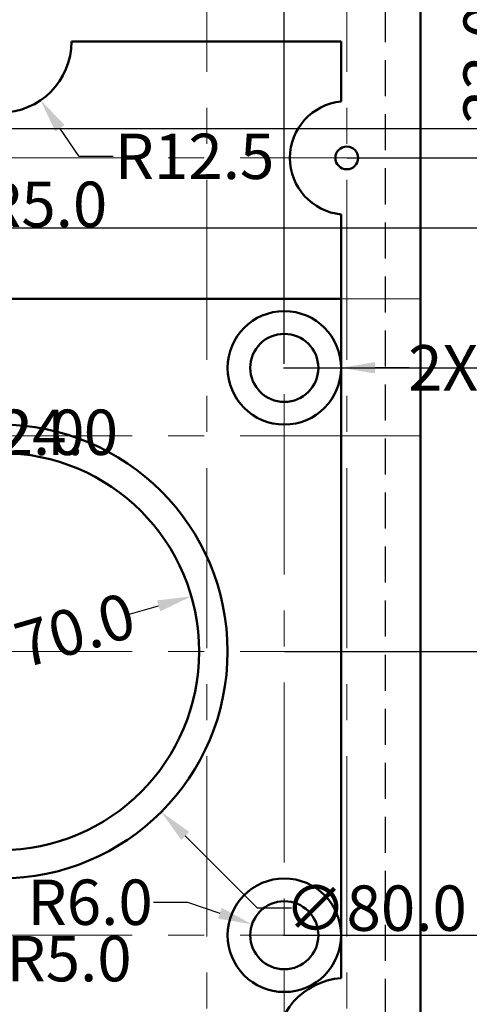
# Model space of a CAD drawing. Units: inches. Extents: x 11765 to 12471, y 10149 to 10793.
# Tile 5 of 8: x 11996 to 12076, y 10530 to 10704. Entities that reach past the tile are written whole.
import ezdxf

# ---------------------------------------------------------------- set-up
doc = ezdxf.new("R2010")
doc.units = ezdxf.units.IN
doc.header["$MEASUREMENT"] = 0
doc.linetypes.add('CENTER', pattern=[50.8, 31.75, -6.35, 6.35, -6.35])
doc.linetypes.add('HIDDEN', pattern=[9.525, 6.35, -3.175])
for name, color, linetype, lineweight in [('M-CNTR', 30, 'CENTER', 18), ('M-DIMS', 2, 'Continuous', 25), ('M-HIDN', 41, 'HIDDEN', 25), ('M-OUTL', 7, 'Continuous', 50)]:
    doc.layers.add(name, color=color, linetype=linetype, lineweight=lineweight)
doc.styles.get("Standard").update_dxf_attribs({"font": 'arial.ttf'})
doc.dimstyles.get("Standard").update_dxf_attribs({"dimtxt": 8, "dimasz": 6, "dimexe": 0.18, "dimexo": 0.0625, "dimgap": 0.09, "dimtad": 0, "dimtoh": 1, "dimdec": 1, "dimzin": 0, "dimdsep": 46, "dimtxsty": 'Standard', "dimcen": 0.09, "dimadec": 0, "dimazin": 0, "dimtfac": 1, "dimtdec": 1, "dimtofl": 0, "dimtmove": 0, "dimatfit": 3, "dimfxl": 1, "dimtolj": 1, "dimtzin": 0, "dimarcsym": 0})

# ---------------------------------------------------------------- blocks, each defined once
blk = doc.blocks.new('*D5')
at = {"layer": 'Defpoints', "color": 0, "transparency": 16777216}
for p in [(11992.91, 10750.5), (11992.91, 10699.65), (12042.91, 10642.79)]:
    blk.add_point(p, dxfattribs=at)
at = {"layer": 'M-DIMS', "color": 0, "lineweight": -2, "transparency": 16777216}
for p, q in [((11992.91, 10699.71), (11992.91, 10750.68)), ((11998.91, 10750.5), (12007.45, 10750.5)), ((12036.91, 10750.5), (12028.38, 10750.5)), ((12042.91, 10642.86), (12042.91, 10750.68))]:
    blk.add_line(p, q, dxfattribs=at)
at = {"layer": 'M-DIMS', "color": 0, "transparency": 16777216}
for points in [[(11998.91, 10751.5), (11998.91, 10749.5), (11992.91, 10750.5)], [(12036.91, 10751.5), (12036.91, 10749.5), (12042.91, 10750.5)]]:
    blk.add_solid(points, dxfattribs=at)
at = {"layer": 'M-DIMS', "color": 0, "transparency": 16777216, "insert": (12017.91, 10750.5), "char_height": 8, "attachment_point": 5}
blk.add_mtext('\\A1;50.0', dxfattribs=at)
blk = doc.blocks.new('*D7')
at = {"layer": 'Defpoints', "color": 0, "transparency": 16777216}
for p in [(12066.91, 10679.15), (12145.22, 10679.15), (12066.91, 10592.15)]:
    blk.add_point(p, dxfattribs=at)
at = {"layer": 'M-DIMS', "color": 0, "lineweight": -2, "transparency": 16777216}
for p, q in [((12066.97, 10679.15), (12145.4, 10679.15)), ((12145.22, 10673.15), (12145.22, 10646.12)), ((12145.22, 10598.15), (12145.22, 10625.17)), ((12066.97, 10592.15), (12145.4, 10592.15))]:
    blk.add_line(p, q, dxfattribs=at)
at = {"layer": 'M-DIMS', "color": 0, "transparency": 16777216}
for points in [[(12144.22, 10673.15), (12146.22, 10673.15), (12145.22, 10679.15)], [(12144.22, 10598.15), (12146.22, 10598.15), (12145.22, 10592.15)]]:
    blk.add_solid(points, dxfattribs=at)
at = {"layer": 'M-DIMS', "color": 0, "transparency": 16777216, "insert": (12145.22, 10635.65), "char_height": 8, "attachment_point": 5, "rotation": 90}
blk.add_mtext('\\A1;87.0', dxfattribs=at)
blk = doc.blocks.new('*D8')
at = {"layer": 'Defpoints', "color": 0, "transparency": 16777216}
for p in [(12042.91, 10642.15), (12042.91, 10592.15), (12085.66, 10592.15)]:
    blk.add_point(p, dxfattribs=at)
at = {"layer": 'M-DIMS', "color": 0, "lineweight": -2, "transparency": 16777216}
for p, q in [((12042.97, 10642.15), (12085.84, 10642.15)), ((12085.66, 10636.15), (12085.66, 10627.61)), ((12085.66, 10598.15), (12085.66, 10606.68)), ((12042.97, 10592.15), (12085.84, 10592.15))]:
    blk.add_line(p, q, dxfattribs=at)
at = {"layer": 'M-DIMS', "color": 0, "transparency": 16777216}
for points in [[(12084.66, 10636.15), (12086.66, 10636.15), (12085.66, 10642.15)], [(12084.66, 10598.15), (12086.66, 10598.15), (12085.66, 10592.15)]]:
    blk.add_solid(points, dxfattribs=at)
at = {"layer": 'M-DIMS', "color": 0, "transparency": 16777216, "insert": (12085.66, 10617.15), "char_height": 8, "attachment_point": 5, "rotation": 90}
blk.add_mtext('\\A1;50.0', dxfattribs=at)
blk = doc.blocks.new('*D9')
at = {"layer": 'Defpoints', "color": 0, "transparency": 16777216}
for p in [(12042.91, 10592.15), (12085.66, 10592.15), (12042.91, 10542.15)]:
    blk.add_point(p, dxfattribs=at)
at = {"layer": 'M-DIMS', "color": 0, "lineweight": -2, "transparency": 16777216}
for p, q in [((12042.97, 10592.15), (12085.84, 10592.15)), ((12085.66, 10586.15), (12085.66, 10577.61)), ((12085.66, 10548.15), (12085.66, 10556.68)), ((12042.97, 10542.15), (12085.84, 10542.15))]:
    blk.add_line(p, q, dxfattribs=at)
at = {"layer": 'M-DIMS', "color": 0, "transparency": 16777216}
for points in [[(12084.66, 10586.15), (12086.66, 10586.15), (12085.66, 10592.15)], [(12084.66, 10548.15), (12086.66, 10548.15), (12085.66, 10542.15)]]:
    blk.add_solid(points, dxfattribs=at)
at = {"layer": 'M-DIMS', "color": 0, "transparency": 16777216, "insert": (12085.66, 10567.15), "char_height": 8, "attachment_point": 5, "rotation": 90}
blk.add_mtext('\\A1;50.0', dxfattribs=at)
blk = doc.blocks.new('*D12')
at = {"layer": 'Defpoints', "color": 0, "transparency": 16777216}
for p in [(12130.14, 10592.15), (12029.23, 10443.15), (12167.12, 10443.15)]:
    blk.add_point(p, dxfattribs=at)
at = {"layer": 'M-DIMS', "color": 0, "lineweight": -2, "transparency": 16777216}
for p, q in [((12130.2, 10592.15), (12167.3, 10592.15)), ((12167.12, 10586.15), (12167.12, 10530.84)), ((12167.12, 10449.15), (12167.12, 10504.45)), ((12029.29, 10443.15), (12167.3, 10443.15))]:
    blk.add_line(p, q, dxfattribs=at)
at = {"layer": 'M-DIMS', "color": 0, "transparency": 16777216}
for points in [[(12166.12, 10586.15), (12168.12, 10586.15), (12167.12, 10592.15)], [(12166.12, 10449.15), (12168.12, 10449.15), (12167.12, 10443.15)]]:
    blk.add_solid(points, dxfattribs=at)
at = {"layer": 'M-DIMS', "color": 0, "transparency": 16777216, "insert": (12167.12, 10517.65), "char_height": 8, "attachment_point": 5, "rotation": 90}
blk.add_mtext('\\A1;149.0', dxfattribs=at)
blk = doc.blocks.new('*D14')
at = {"layer": 'Defpoints', "color": 0, "transparency": 16777216}
for p in [(12156.23, 10592.15), (12216.5, 10592.15), (11992.91, 10372.15)]:
    blk.add_point(p, dxfattribs=at)
at = {"layer": 'M-DIMS', "color": 0, "lineweight": -2, "transparency": 16777216}
for p, q in [((12156.3, 10592.15), (12216.68, 10592.15)), ((12216.5, 10586.15), (12216.5, 10495.79)), ((12216.5, 10378.15), (12216.5, 10468.5)), ((11992.97, 10372.15), (12216.68, 10372.15))]:
    blk.add_line(p, q, dxfattribs=at)
at = {"layer": 'M-DIMS', "color": 0, "transparency": 16777216}
for points in [[(12215.5, 10586.15), (12217.5, 10586.15), (12216.5, 10592.15)], [(12215.5, 10378.15), (12217.5, 10378.15), (12216.5, 10372.15)]]:
    blk.add_solid(points, dxfattribs=at)
at = {"layer": 'M-DIMS', "color": 0, "transparency": 16777216, "insert": (12216.5, 10482.15), "char_height": 8, "attachment_point": 5, "rotation": 90}
blk.add_mtext('\\A1;220.0', dxfattribs=at)
blk = doc.blocks.new('*D28')
at = {"layer": 'Defpoints', "color": 0, "transparency": 16777216}
for p in [(12053.91, 10712.15), (12078.49, 10712.15), (12053.91, 10679.15)]:
    blk.add_point(p, dxfattribs=at)
at = {"layer": 'M-DIMS', "color": 0, "lineweight": -2, "transparency": 16777216}
for p, q in [((12078.49, 10718.15), (12078.49, 10724.15)), ((12053.97, 10712.15), (12078.67, 10712.15)), ((12053.97, 10679.15), (12078.67, 10679.15)), ((12078.49, 10673.15), (12078.49, 10667.15))]:
    blk.add_line(p, q, dxfattribs=at)
at = {"layer": 'M-DIMS', "color": 0, "transparency": 16777216}
for points in [[(12077.49, 10718.15), (12079.49, 10718.15), (12078.49, 10712.15)], [(12077.49, 10673.15), (12079.49, 10673.15), (12078.49, 10679.15)]]:
    blk.add_solid(points, dxfattribs=at)
at = {"layer": 'M-DIMS', "color": 0, "transparency": 16777216, "insert": (12078.49, 10695.65), "char_height": 8, "attachment_point": 5, "rotation": 90}
blk.add_mtext('\\A1;33.0', dxfattribs=at)
blk = doc.blocks.new('*D33')
at = {"layer": 'Defpoints', "color": 0, "transparency": 16777216}
for p in [(11992.91, 10699.65), (11999.97, 10689.33)]:
    blk.add_point(p, dxfattribs=at)
at = {"layer": 'M-DIMS', "color": 0, "lineweight": -2, "transparency": 16777216}
for p, q in [((11992.82, 10699.65), (11993, 10699.65)), ((11992.91, 10699.56), (11992.91, 10699.74)), ((12006.75, 10679.43), (12003.36, 10684.38)), ((12012.75, 10679.43), (12006.75, 10679.43))]:
    blk.add_line(p, q, dxfattribs=at)
at = {"layer": 'M-DIMS', "color": 0, "transparency": 16777216}
blk.add_solid([(12004.19, 10684.95), (12002.54, 10683.82), (11999.97, 10689.33)], dxfattribs=at)
at = {"layer": 'M-DIMS', "color": 0, "transparency": 16777216, "insert": (12027.09, 10679.43), "char_height": 8, "attachment_point": 5}
blk.add_mtext('\\A1;R12.5', dxfattribs=at)
blk = doc.blocks.new('*D34')
at = {"layer": 'Defpoints', "color": 0, "transparency": 16777216}
for p in [(11969.55, 10659.29), (11965.72, 10656.07)]:
    blk.add_point(p, dxfattribs=at)
at = {"layer": 'M-DIMS', "color": 0, "lineweight": -2, "transparency": 16777216}
for p, q in [((11983.49, 10670.97), (11970.32, 10659.93)), ((11989.49, 10670.97), (11983.49, 10670.97))]:
    blk.add_line(p, q, dxfattribs=at)
at = {"layer": 'M-DIMS', "color": 0, "transparency": 16777216}
blk.add_solid([(11969.68, 10660.69), (11970.96, 10659.16), (11965.72, 10656.07)], dxfattribs=at)
at = {"layer": 'M-DIMS', "color": 0, "transparency": 16777216, "insert": (12000.68, 10670.97), "char_height": 8, "attachment_point": 5}
blk.add_mtext('\\A1;R5.0', dxfattribs=at)
blk = doc.blocks.new('*D41')
at = {"layer": 'Defpoints', "color": 0, "transparency": 16777216}
for p in [(11987.78, 10526.02), (11987.78, 10521.02)]:
    blk.add_point(p, dxfattribs=at)
at = {"layer": 'M-DIMS', "color": 0, "lineweight": -2, "transparency": 16777216}
for p, q in [((11993.78, 10538.02), (11987.78, 10538.02)), ((11987.78, 10538.02), (11987.78, 10532.02)), ((11987.69, 10521.02), (11987.87, 10521.02)), ((11987.78, 10520.93), (11987.78, 10521.11))]:
    blk.add_line(p, q, dxfattribs=at)
at = {"layer": 'M-DIMS', "color": 0, "transparency": 16777216}
blk.add_solid([(11986.78, 10532.02), (11988.78, 10532.02), (11987.78, 10526.02)], dxfattribs=at)
at = {"layer": 'M-DIMS', "color": 0, "transparency": 16777216, "insert": (12004.97, 10538.02), "char_height": 8, "attachment_point": 5}
blk.add_mtext('\\A1;R5.0', dxfattribs=at)
blk = doc.blocks.new('*D42')
at = {"layer": 'Defpoints', "color": 0, "transparency": 16777216}
for p in [(12026.53, 10601.87), (11959.29, 10582.42)]:
    blk.add_point(p, dxfattribs=at)
at = {"layer": 'M-DIMS', "color": 0, "lineweight": -2, "transparency": 16777216}
blk.add_line((12015.01, 10598.54), (12020.77, 10600.2), dxfattribs=at)
at = {"layer": 'M-DIMS', "color": 0, "transparency": 16777216}
blk.add_solid([(12020.49, 10601.16), (12021.05, 10599.24), (12026.53, 10601.87)], dxfattribs=at)
at = {"layer": 'M-DIMS', "color": 0, "transparency": 16777216, "insert": (12000.77, 10594.42), "char_height": 8, "attachment_point": 5, "rotation": 16.1306}
blk.add_mtext('\\A1;∅70.0', dxfattribs=at)
blk = doc.blocks.new('*D43')
at = {"layer": 'Defpoints', "color": 0, "transparency": 16777216}
for p in [(11953.39, 10598.33), (12032.43, 10585.96)]:
    blk.add_point(p, dxfattribs=at)
at = {"layer": 'M-DIMS', "color": 0, "lineweight": -2, "transparency": 16777216}
for p, q in [((11927.12, 10602.44), (11947.47, 10599.26)), ((11992.82, 10592.15), (11993, 10592.15)), ((11992.91, 10592.06), (11992.91, 10592.24))]:
    blk.add_line(p, q, dxfattribs=at)
at = {"layer": 'M-DIMS', "color": 0, "transparency": 16777216}
blk.add_solid([(11947.62, 10600.25), (11947.31, 10598.27), (11953.39, 10598.33)], dxfattribs=at)
at = {"layer": 'M-DIMS', "color": 0, "transparency": 16777216, "insert": (11912.3, 10602.44), "char_height": 8, "attachment_point": 5}
blk.add_mtext('\\A1;∅80.0', dxfattribs=at)
blk = doc.blocks.new('*D49')
at = {"layer": 'Defpoints', "color": 0, "transparency": 16777216}
for p in [(12037.23, 10544.08), (12042.91, 10542.15)]:
    blk.add_point(p, dxfattribs=at)
at = {"layer": 'M-DIMS', "color": 0, "lineweight": -2, "transparency": 16777216}
for p, q in [((12019.88, 10547.96), (12025.88, 10547.96)), ((12025.88, 10547.96), (12031.55, 10546.02)), ((12042.82, 10542.15), (12043, 10542.15)), ((12042.91, 10542.06), (12042.91, 10542.24))]:
    blk.add_line(p, q, dxfattribs=at)
at = {"layer": 'M-DIMS', "color": 0, "transparency": 16777216}
blk.add_solid([(12031.88, 10546.97), (12031.23, 10545.07), (12037.23, 10544.08)], dxfattribs=at)
at = {"layer": 'M-DIMS', "color": 0, "transparency": 16777216, "insert": (12008.69, 10547.96), "char_height": 8, "attachment_point": 5}
blk.add_mtext('\\A1;R6.0', dxfattribs=at)
blk = doc.blocks.new('*D62')
at = {"layer": 'Defpoints', "color": 0, "transparency": 16777216}
for p in [(12379.9, 10706.15), (11848.16, 10684.29), (12385.4, 10684.29)]:
    blk.add_point(p, dxfattribs=at)
at = {"layer": 'M-DIMS', "color": 0, "lineweight": -2, "transparency": 16777216}
for p, q in [((12379.83, 10706.15), (11847.98, 10706.15)), ((11848.16, 10700.15), (11848.16, 10690.29)), ((12385.33, 10684.29), (11847.98, 10684.29)), ((11848.16, 10684.29), (11848.16, 10678.29)), ((11848.16, 10678.29), (11842.16, 10678.29))]:
    blk.add_line(p, q, dxfattribs=at)
at = {"layer": 'M-DIMS', "color": 0, "transparency": 16777216}
for points in [[(11847.16, 10700.15), (11849.16, 10700.15), (11848.16, 10706.15)], [(11847.16, 10690.29), (11849.16, 10690.29), (11848.16, 10684.29)]]:
    blk.add_solid(points, dxfattribs=at)
at = {"layer": 'M-DIMS', "color": 0, "transparency": 16777216, "insert": (11828.51, 10678.29), "char_height": 8, "attachment_point": 5}
blk.add_mtext('\\A1;21.86', dxfattribs=at)
blk = doc.blocks.new('*D63')
at = {"layer": 'Defpoints', "color": 0, "transparency": 16777216}
for p in [(12385.4, 10684.29), (11848.16, 10666.79), (12385.4, 10666.79)]:
    blk.add_point(p, dxfattribs=at)
at = {"layer": 'M-DIMS', "color": 0, "lineweight": -2, "transparency": 16777216}
for p, q in [((12385.33, 10684.29), (11847.98, 10684.29)), ((11848.16, 10678.29), (11848.16, 10672.79)), ((12385.33, 10666.79), (11847.98, 10666.79)), ((11848.16, 10666.79), (11848.16, 10660.79)), ((11848.16, 10660.79), (11842.16, 10660.79))]:
    blk.add_line(p, q, dxfattribs=at)
at = {"layer": 'M-DIMS', "color": 0, "transparency": 16777216}
for points in [[(11847.16, 10678.29), (11849.16, 10678.29), (11848.16, 10684.29)], [(11847.16, 10672.79), (11849.16, 10672.79), (11848.16, 10666.79)]]:
    blk.add_solid(points, dxfattribs=at)
at = {"layer": 'M-DIMS', "color": 0, "transparency": 16777216, "insert": (11832.03, 10660.79), "char_height": 8, "attachment_point": 5}
blk.add_mtext('\\A1;17.5', dxfattribs=at)
blk = doc.blocks.new('*D68')
at = {"layer": 'Defpoints', "color": 0, "transparency": 16777216}
for p in [(11964.61, 10620.41), (12021.22, 10563.88)]:
    blk.add_point(p, dxfattribs=at)
at = {"layer": 'M-DIMS', "color": 0, "lineweight": -2, "transparency": 16777216}
for p, q in [((11992.82, 10592.15), (11993, 10592.15)), ((11992.91, 10592.06), (11992.91, 10592.24)), ((12038.2, 10546.92), (12025.46, 10559.64)), ((12044.2, 10546.92), (12038.2, 10546.92))]:
    blk.add_line(p, q, dxfattribs=at)
at = {"layer": 'M-DIMS', "color": 0, "transparency": 16777216}
blk.add_solid([(12026.17, 10560.35), (12024.76, 10558.94), (12021.22, 10563.88)], dxfattribs=at)
at = {"layer": 'M-DIMS', "color": 0, "transparency": 16777216, "insert": (12059.02, 10546.92), "char_height": 8, "attachment_point": 5}
blk.add_mtext('\\A1;∅80.0', dxfattribs=at)
blk = doc.blocks.new('*D69')
at = {"layer": 'Defpoints', "color": 0, "transparency": 16777216}
for p in [(11968.18, 10616.92), (12017.64, 10567.38)]:
    blk.add_point(p, dxfattribs=at)
at = {"layer": 'M-DIMS', "color": 0, "lineweight": -2, "transparency": 16777216}
for p, q in [((11947.35, 10631.78), (11953.35, 10631.78)), ((11953.35, 10631.78), (11963.95, 10621.16)), ((11992.82, 10592.15), (11993, 10592.15)), ((11992.91, 10592.06), (11992.91, 10592.24))]:
    blk.add_line(p, q, dxfattribs=at)
at = {"layer": 'M-DIMS', "color": 0, "transparency": 16777216}
blk.add_solid([(11964.65, 10621.87), (11963.24, 10620.46), (11968.18, 10616.92)], dxfattribs=at)
at = {"layer": 'M-DIMS', "color": 0, "transparency": 16777216, "insert": (11932.53, 10631.78), "char_height": 8, "attachment_point": 5}
blk.add_mtext('\\A1;∅70.0', dxfattribs=at)
blk = doc.blocks.new('*D78')
at = {"layer": 'Defpoints', "color": 0, "transparency": 16777216}
for p in [(11930.91, 10630.79), (11954.91, 10630.79)]:
    blk.add_point(p, dxfattribs=at)
at = {"layer": 'M-DIMS', "color": 0, "lineweight": -2, "transparency": 16777216}
for p, q in [((11942.82, 10630.79), (11943, 10630.79)), ((11942.91, 10630.7), (11942.91, 10630.88)), ((11966.91, 10630.79), (11960.91, 10630.79))]:
    blk.add_line(p, q, dxfattribs=at)
at = {"layer": 'M-DIMS', "color": 0, "transparency": 16777216}
blk.add_solid([(11960.91, 10631.79), (11960.91, 10629.79), (11954.91, 10630.79)], dxfattribs=at)
at = {"layer": 'M-DIMS', "color": 0, "transparency": 16777216, "insert": (11990.18, 10630.79), "char_height": 8, "attachment_point": 5}
blk.add_mtext('\\A1;2X ∅24.0', dxfattribs=at)
blk = doc.blocks.new('*D80')
at = {"layer": 'Defpoints', "color": 0, "transparency": 16777216}
for p in [(12032.91, 10642.15), (12052.91, 10642.15)]:
    blk.add_point(p, dxfattribs=at)
at = {"layer": 'M-DIMS', "color": 0, "lineweight": -2, "transparency": 16777216}
for p, q in [((12042.82, 10642.15), (12043, 10642.15)), ((12042.91, 10642.06), (12042.91, 10642.24)), ((12064.91, 10642.15), (12058.91, 10642.15))]:
    blk.add_line(p, q, dxfattribs=at)
at = {"layer": 'M-DIMS', "color": 0, "transparency": 16777216}
blk.add_solid([(12058.91, 10643.15), (12058.91, 10641.15), (12052.91, 10642.15)], dxfattribs=at)
at = {"layer": 'M-DIMS', "color": 0, "transparency": 16777216, "insert": (12088.18, 10642.15), "char_height": 8, "attachment_point": 5}
blk.add_mtext('\\A1;2X ∅20.0', dxfattribs=at)
blk = doc.blocks.new('*D81')
at = {"layer": 'Defpoints', "color": 0, "transparency": 16777216}
for p in [(11936.91, 10630.79), (11948.91, 10630.79)]:
    blk.add_point(p, dxfattribs=at)
at = {"layer": 'M-DIMS', "color": 0, "lineweight": -2, "transparency": 16777216}
for p, q in [((11942.82, 10630.79), (11943, 10630.79)), ((11942.91, 10630.7), (11942.91, 10630.88)), ((11960.91, 10630.79), (11954.91, 10630.79))]:
    blk.add_line(p, q, dxfattribs=at)
at = {"layer": 'M-DIMS', "color": 0, "transparency": 16777216}
blk.add_solid([(11954.91, 10631.79), (11954.91, 10629.79), (11948.91, 10630.79)], dxfattribs=at)
at = {"layer": 'M-DIMS', "color": 0, "transparency": 16777216, "insert": (11984.27, 10630.79), "char_height": 8, "attachment_point": 5}
blk.add_mtext('\\A1;4X ∅12.0', dxfattribs=at)

msp = doc.modelspace()

# ---------------------------------------------------------------- linework, layer by layer
at = {"layer": 'M-CNTR'}
for p, q in [((12029.232, 10237.146), (12029.232, 10712.146)), ((12042.912, 10504.146), (12042.912, 10712.146)), ((12053.912, 10237.146), (12053.912, 10712.146)), ((12066.912, 10679.146), (11882.912, 10679.146)), ((12066.912, 10654.286), (11882.912, 10654.286)), ((12066.912, 10630.146), (11882.912, 10630.146)), ((12066.912, 10592.146), (11882.912, 10592.146)), ((12066.912, 10542.146), (11882.912, 10542.146))]:
    msp.add_line(p, q, dxfattribs=at)
at = {"layer": 'M-HIDN'}
msp.add_lwpolyline([(12060.662, 10705.896), (12060.662, 10515.896), (12096.662, 10515.896), (12096.662, 10263.352), (12062.096, 10243.396), (11923.728, 10243.396), (11889.162, 10263.352), (11889.162, 10705.896)], close=True, dxfattribs=at)
at = {"layer": 'M-OUTL'}
for p, q in [((12066.912, 10522.146), (12066.912, 10712.146)), ((12052.912, 10699.646), (12005.412, 10699.646)), ((12052.912, 10699.646), (12052.912, 10689.095)), ((12052.912, 10669.196), (12052.912, 10534.605)), ((11969.553, 10654.286), (12052.912, 10654.286))]:
    msp.add_line(p, q, dxfattribs=at)
for centre, radius in [((12053.912, 10679.146), 2), ((12042.912, 10642.146), 10), ((12042.912, 10642.146), 6), ((11992.912, 10592.146), 40), ((11992.912, 10592.146), 35), ((12042.912, 10542.146), 10), ((12042.912, 10542.146), 6)]:
    msp.add_circle(centre, radius, dxfattribs=at)
for centre, radius, start, end in [((11992.912, 10699.646), 12.5, 270, 0), ((12053.912, 10679.146), 10, 95.73917, 264.26083), ((12053.912, 10522.146), 12.5, 94.58857, 270)]:
    msp.add_arc(centre, radius, start, end, dxfattribs=at)

# ---------------------------------------------------------------- dimensions: what is measured, and where the dimension line sits
at = {"layer": 'M-DIMS'}
dim = msp.add_linear_dim(base=(11992.912, 10750.499), p1=(12042.912, 10642.793), p2=(11992.912, 10699.646), dimstyle='Standard', override={"dimclrd": 0, "dimclre": 0, "dimclrt": 0}, dxfattribs=at)
dim.commit()
dim.dimension.update_dxf_attribs({"geometry": '*D5', "text_midpoint": (12017.912, 10750.499)})
for base, p1, p2, override, picture, middle in [((12078.487, 10712.146), (12053.912, 10679.146), (12053.912, 10712.146), {"dimclrd": 0, "dimclre": 0, "dimclrt": 0}, '*D28', (12078.487, 10695.646)), ((11848.162, 10684.286), (12379.896, 10706.146), (12385.396, 10684.286), {"dimdec": 2, "dimlfac": 1, "dimrnd": 0, "dimzin": 0, "dimdsep": 46, "dimlunit": 2}, '*D62', (11828.509, 10678.286)), ((11848.162, 10666.786), (12385.396, 10684.286), (12385.396, 10666.786), {"dimdec": 1, "dimlfac": 1, "dimrnd": 0, "dimzin": 0, "dimdsep": 46, "dimlunit": 2}, '*D63', (11832.028, 10660.786)), ((12145.224, 10679.146), (12066.912, 10592.146), (12066.912, 10679.146), {"dimclrd": 0, "dimclre": 0, "dimclrt": 0}, '*D7', (12145.224, 10635.646)), ((12085.657, 10592.146), (12042.912, 10642.146), (12042.912, 10592.146), {"dimclrd": 0, "dimclre": 0, "dimclrt": 0}, '*D8', (12085.657, 10617.146)), ((12216.505, 10592.146), (11992.912, 10372.146), (12156.234, 10592.146), {"dimclrd": 0, "dimclre": 0, "dimclrt": 0}, '*D14', (12216.505, 10482.146)), ((12167.122, 10443.146), (12130.138, 10592.146), (12029.232, 10443.146), {"dimclrd": 0, "dimclre": 0, "dimclrt": 0}, '*D12', (12167.122, 10517.646)), ((12085.657, 10592.146), (12042.912, 10542.146), (12042.912, 10592.146), {"dimclrd": 0, "dimclre": 0, "dimclrt": 0}, '*D9', (12085.657, 10567.146))]:
    dim = msp.add_linear_dim(base=base, p1=p1, p2=p2, angle=90, dimstyle='Standard', override=override, dxfattribs=at)
    dim.commit()
    dim.dimension.update_dxf_attribs({"geometry": picture, "text_midpoint": middle})
for center, mpoint, picture, middle in [((11992.912, 10699.646), (11999.974, 10689.332), '*D33', (12027.093, 10679.431)), ((12042.912, 10542.146), (12037.233, 10544.082), '*D49', (12008.689, 10547.956)), ((11987.783, 10521.025), (11987.783, 10526.025), '*D41', (12004.97, 10538.025))]:
    dim = msp.add_radius_dim(center=center, mpoint=mpoint, dimstyle='Standard', override={"dimclrd": 0, "dimclre": 0, "dimclrt": 0}, dxfattribs=at)
    dim.commit()
    dim.dimension.update_dxf_attribs({"geometry": picture, "text_midpoint": middle})
dim = msp.add_radius_dim(center=(11969.553, 10659.286), mpoint=(11965.721, 10656.074), dimstyle='Standard', override={"dimclrd": 0, "dimclre": 0, "dimclrt": 0}, dxfattribs=at)
dim.commit()
dim.dimension.update_dxf_attribs({"geometry": '*D34', "text_midpoint": (12000.68, 10670.966), "dimtype": 164})
dim = msp.add_diameter_dim_2p(p1=(12032.912, 10642.145), p2=(12052.912, 10642.146), text='2X <>', dimstyle='Standard', override={"dimdec": 1, "dimlfac": 1, "dimrnd": 0, "dimzin": 0, "dimdsep": 46, "dimlunit": 2}, dxfattribs=at)
dim.commit()
dim.dimension.update_dxf_attribs({"geometry": '*D80', "text_midpoint": (12064.912, 10642.147)})
for p1, p2, text, picture, middle in [((11930.912, 10630.793), (11954.912, 10630.793), '2X <>', '*D78', (11966.912, 10630.793)), ((11936.912, 10630.793), (11948.912, 10630.793), '4X <>', '*D81', (11960.912, 10630.793))]:
    dim = msp.add_diameter_dim_2p(p1=p1, p2=p2, text=text, dimstyle='Standard', override={"dimdec": 1, "dimlfac": 1, "dimrnd": 0, "dimzin": 0, "dimdsep": 46, "dimlunit": 2}, dxfattribs=at)
    dim.commit()
    dim.dimension.update_dxf_attribs({"geometry": picture, "text_midpoint": middle, "dimtype": 163})
for p1, p2, override, picture, middle in [((12017.639, 10567.376), (11968.185, 10616.916), {"dimdec": 1, "dimlfac": 1, "dimrnd": 0, "dimzin": 0, "dimdsep": 46, "dimlunit": 2}, '*D69', (11932.529, 10631.777)), ((11964.607, 10620.409), (12021.217, 10563.883), {"dimdec": 1, "dimlfac": 1, "dimrnd": 0, "dimzin": 0, "dimdsep": 46, "dimlunit": 2}, '*D68', (12059.019, 10546.925)), ((12032.431, 10585.96), (11953.393, 10598.331), {"dimclrd": 0, "dimclre": 0, "dimclrt": 0}, '*D43', (11927.122, 10602.444)), ((11959.29, 10582.422), (12026.534, 10601.87), {"dimclrd": 0, "dimclre": 0, "dimclrt": 0}, '*D42', (12000.771, 10594.419))]:
    dim = msp.add_diameter_dim_2p(p1=p1, p2=p2, dimstyle='Standard', override=override, dxfattribs=at)
    dim.commit()
    dim.dimension.update_dxf_attribs({"geometry": picture, "text_midpoint": middle, "dimtype": 163})

doc.saveas('drawing.dxf')
